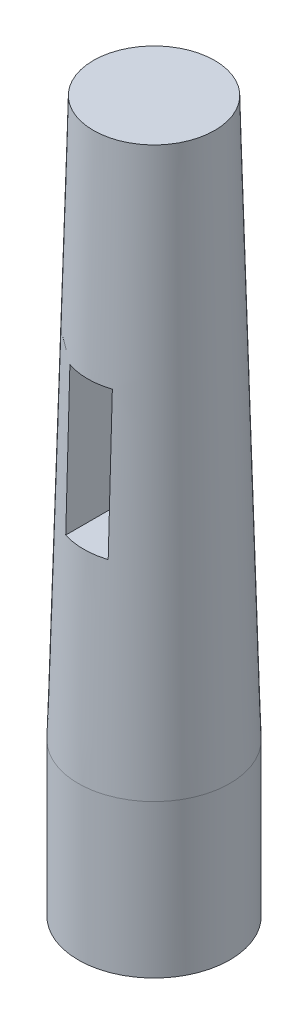
SolidWorks part; units mm, degrees
material "Plain Carbon Steel"
ref_plane "Front Plane" through (0, 0, 0) normal (0, 0, 1) x (1, 0, 0)
ref_plane "Top Plane" through (0, 0, 0) normal (0, 1, 0) x (1, 0, 0)
ref_plane "Right Plane" through (0, 0, 0) normal (1, 0, 0) x (0, 0, -1)
sketch "Base Shank Profile Ø25.2" plane through (0, 0, 0) normal (0, 1, 0) x (1, 0, 0)
  circle A0 centre (0, 0) radius 12.5
  dimension "D1" = 25
extrude "Base Shank Ø25.2" add sketch "Base Shank Profile Ø25.2" along normal blind 25.2
sketch "Taper Start Profile Ø25.2" plane through (0, 25.2, 0) normal (0, 1, 0) x (1, 0, 0)
  circle A0 centre (0, 0) radius 12.5
  dimension "D1" = 25
ref_plane "Taper End Plane" through (0, 117.2, 0) normal (0, 1, 0) x (1, 0, 0)
sketch "Taper End Profile Ø20.2" plane through (0, 117.2, 0) normal (0, 1, 0) x (1, 0, 0)
  circle A0 centre (0, 0) radius 10
  dimension "D1" = 20
loft "Tapered Rod Loft" add profiles "Taper Start Profile Ø25.2", "Taper End Profile Ø20.2"
sketch "Through Slot Profile" plane through (0, 0, 0) normal (0, 0, 1) x (1, 0, 0)
  line L0 (12.5, 25.2) -> (-12.5, 25.2) construction
  line L1 (-3.5, 82.2) -> (3.5, 82.2)
  line L2 (-3.5, 82.2) -> (-3.5, 58.2)
  line L3 (-3.5, 58.2) -> (3.5, 58.2)
  line L4 (3.5, 82.2) -> (3.5, 58.2)
  line L5 (-3.5, 82.2) -> (3.5, 58.2) construction
  line L6 (-3.5, 58.2) -> (3.5, 82.2) construction
  point P0 (0, 70.2)
  dimension "D1" = 33
  dimension "D2" = 24
  dimension "D3" = 7
extrude "Through Slot" cut sketch "Through Slot Profile" against normal mid plane 35.2
